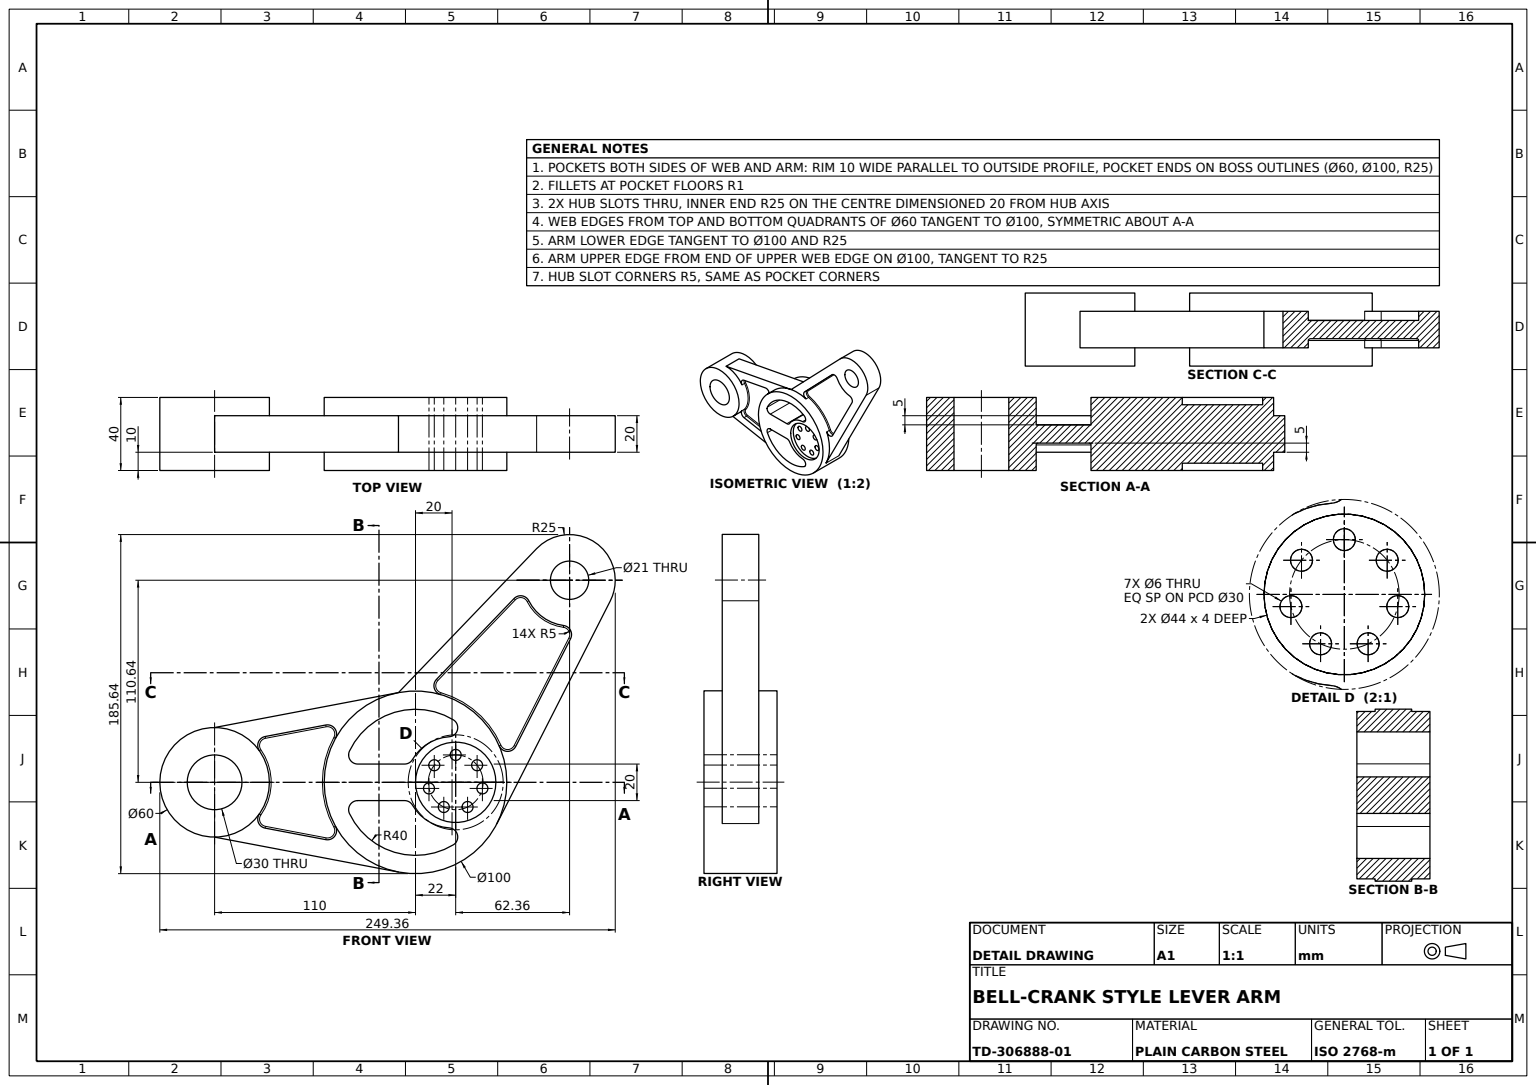
SolidWorks part; units mm, degrees
material "Plain Carbon Steel"
ref_plane "Front Plane" through (0, 0, 0) normal (0, 0, 1) x (1, 0, 0)
ref_plane "Top Plane" through (0, 0, 0) normal (0, 1, 0) x (1, 0, 0)
ref_plane "Right Plane" through (0, 0, 0) normal (1, 0, 0) x (0, 0, -1)
sketch "Lever Body Profile" plane through (0, 0, 0) normal (0, 0, 1) x (1, 0, 0)
  line L0 (0, 0) -> (-50, 0)
  line L1 (-5.9808, 10) -> (-31.6228, 10)
  line L2 (-5.9808, -10) -> (-31.6228, -10)
  line L4 (0, 10) -> (-50, 10) construction
  circle A0 centre (0, 0) radius 50
  arc A1 (20.7143, 34.2187) -> (-36.1403, 17.1429) centre (0, 0) ccw
  arc A4 (18.4375, 24.9511) -> (-1.6506, 12.5) centre (20, 0) ccw
  arc A5 (18.4375, 24.9511) -> (20.7143, 34.2187) centre (18.125, 29.9413) ccw
  arc A6 (18.4375, -24.9511) -> (20.7143, -34.2187) centre (18.125, -29.9413) cw
  arc A7 (-5.9808, -10) -> (-1.6506, -12.5) centre (-5.9808, -15) cw
  arc A8 (-5.9808, 10) -> (-1.6506, 12.5) centre (-5.9808, 15) ccw
  arc A9 (-31.6228, 10) -> (-36.1403, 17.1429) centre (-31.6228, 15) cw
  arc A10 (18.4375, -24.9511) -> (-1.6506, -12.5) centre (20, 0) cw
  arc A11 (-31.6228, -10) -> (-36.1403, -17.1429) centre (-31.6228, -15) ccw
  arc A12 (20.7143, -34.2187) -> (-36.1403, -17.1429) centre (0, 0) cw
  point P12 (0, -10)
  point P13 (-50, -10)
  dimension "D1" = 100
  dimension "D2" = 80
  dimension "D3" = 20
  dimension "D5" = 50
  dimension "D6" = 10
  dimension "D7" = 5
  dimension "D8" = 5
extrude "Lever Body" add sketch "Lever Body Profile" along normal blind 40
sketch "Front Pocket Profile" plane through (0, 0, 40) normal (0, 0, 1) x (1, 0, 0)
  line L0 (-5.9808, 10) -> (-31.6228, 10) construction
  circle A0 centre (22, 0) radius 22
  circle A2 centre (22, 15) radius 3
  circle A3 centre (33.7275, 9.3523) radius 3
  circle A4 centre (36.6239, -3.3378) radius 3
  circle A5 centre (28.5083, -13.5145) radius 3
  circle A6 centre (15.4917, -13.5145) radius 3
  circle A7 centre (7.3761, -3.3378) radius 3
  circle A8 centre (10.2725, 9.3523) radius 3
  dimension "D1" = 22
  dimension "D2" = 44
  dimension "D3" = 43.5164
  dimension "D4" = 6
  dimension "D5" = 7
  dimension "D6" = 46.4128
  dimension "D7" = 5
extrude "Front Pocket 4mm" cut sketch "Front Pocket Profile" against normal blind 4
sketch "Hub Through Cut Profile" plane through (0, 0, 40) normal (0, 0, 1) x (1, 0, 0)
  circle A0 centre (22, 15) radius 3
  circle A1 centre (33.7275, 9.3523) radius 3
  circle A2 centre (36.6239, -3.3378) radius 3
  circle A3 centre (28.5083, -13.5145) radius 3
  circle A4 centre (15.4917, -13.5145) radius 3
  circle A5 centre (7.3761, -3.3378) radius 3
  circle A6 centre (10.2725, 9.3523) radius 3
  circle A7 centre (22, 15) radius 3 construction
  dimension "D1" = 7
  dimension "D2" = 6
  dimension "D3" = 6.5083
extrude "Hub Through Cut" cut sketch "Hub Through Cut Profile" against normal blind 44
sketch "Rear Pocket Profile" plane through (0, 0, 0) normal (0, 0, -1) x (-1, 0, 0)
  line L0 (5.9808, 10) -> (31.6228, 10) construction
  circle A7 centre (-22, 0) radius 22
  circle A8 centre (-22, 15) radius 3
  circle A9 centre (-10.2725, 9.3523) radius 3
  circle A10 centre (-7.3761, -3.3378) radius 3
  circle A11 centre (-15.4917, -13.5145) radius 3
  circle A12 centre (-28.5083, -13.5145) radius 3
  circle A13 centre (-36.6239, -3.3378) radius 3
  circle A14 centre (-33.7275, 9.3523) radius 3
  dimension "D1" = 44
  dimension "D2" = 6
  dimension "D3" = 7
  dimension "D4" = 9.0267
  dimension "D5" = 11.9232
  dimension "D6" = 5
  dimension "D8" = 10
extrude "Rear Pocket 4mm" cut sketch "Rear Pocket Profile" against normal blind 4
sketch "Arm Boss Profile" plane through (0, 0, 40) normal (0, 0, 1) x (1, 0, 0)
  circle A0 centre (-110, 0) radius 15
  circle A1 centre (-110, 0) radius 30
  dimension "D1" = 60
  dimension "D2" = 30
  dimension "D3" = 110
  dimension "D4" = 73.8597
extrude "Arm Boss" add sketch "Arm Boss Profile" against normal blind 40 separate body
sketch "Web Arm Profile" plane through (0, 0, 40) normal (0, 0, 1) x (1, 0, 0)
  line L0 (22, 15) -> (22, 0)
  line L1 (-5.9808, 10) -> (-31.6228, 10) construction
  circle A0 centre (84.359, 110.6361) radius 10.5
  circle A1 centre (84.359, 110.6361) radius 25
  dimension "D1" = 21
  dimension "D2" = 50
  dimension "D3" = 127
  dimension "D4" = 62.359
  dimension "D5" = 100.6361
extrude "Triangular Web Arm" add sketch "Web Arm Profile" against normal blind 40 separate body contours A1 A0
ref_plane "Plane1" through (0, 0, 20) normal (0, 0, 1) x (1, 0, 0)
sketch "Front Hub Boss Profile" plane through (0, 0, 20) normal (0, 0, 1) x (1, 0, 0)
  line L0 (-110, 30) -> (-9.3304, 49.1217)
  line L1 (-110, -30) -> (-9.3304, -49.1217)
  line L2 (-9.3304, 49.1217) -> (66.3221, 127.9471)
  line L3 (106.6394, 99.2967) -> (44.5608, -22.6789)
  line L4 (11.4718, 56.3547) -> (53.9518, 100.6162)
  line L5 (84.8981, 78.625) -> (54.8924, 19.668)
  line L6 (-110, 0) -> (0, 0)
  line L7 (-2.1157, 42.1973) -> (73.5368, 121.0227) construction
  line L8 (97.7273, 103.8325) -> (35.6487, -18.1431) construction
  line L9 (-82.3262, 25.0777) -> (-49.1455, 31.3802)
  line L10 (-82.3262, -25.0777) -> (-49.1455, -31.3802)
  line L11 (-108.1339, 20.1757) -> (-7.4644, 39.2974) construction
  arc A0 (-110, 30) -> (-110, -30) centre (-110, 0) cw
  circle A1 centre (-110, 0) radius 30 construction
  circle A2 centre (0, 0) radius 50 construction
  circle A3 centre (0, 0) radius 50
  circle A4 centre (84.359, 110.6361) radius 25 construction
  arc A5 (66.3221, 127.9471) -> (106.6394, 99.2967) centre (84.359, 110.6361) ccw
  arc A6 (11.4718, 56.3547) -> (13.7084, 48.0841) centre (15.0792, 52.8925) ccw
  arc A7 (45.8512, 19.9417) -> (54.8924, 19.668) centre (50.4363, 21.9359) ccw
  arc A8 (53.9518, 100.6162) -> (62.0258, 99.401) centre (57.5591, 97.154) cw
  arc A9 (81.0949, 85.8501) -> (84.8981, 78.625) centre (80.442, 80.8929) cw
  arc A10 (-82.3262, 25.0777) -> (-85.4799, 17.2847) centre (-81.3932, 20.1655) ccw
  arc A11 (-49.1455, 31.3802) -> (-43.8295, 24.0619) centre (-48.2125, 26.4681) cw
  arc A12 (-49.1455, -31.3802) -> (-43.8295, -24.0619) centre (-48.2125, -26.4681) ccw
  arc A13 (-82.3262, -25.0777) -> (-85.4799, -17.2847) centre (-81.3932, -20.1655) cw
  dimension "D1" = 30
  dimension "D2" = 100
  dimension "D6" = 5
  dimension "D7" = 5
  dimension "D8" = 5
  dimension "D9" = 5
  dimension "D11" = 5
  dimension "D12" = 5
  dimension "D10" = 10
  dimension "D4" = 10
  dimension "D5" = 10
extrude "Front Hub Boss" add sketch "Front Hub Boss Profile" along normal mid plane 20 contours L9 A11 A3 L0 A0 A10 | L10 A13 A0 L1 A3 A12 | L4 A8 A5 L2 A3 A6 | A5 A9 L5 A7 A3 L3
ref_plane "Plane2" through (0, 0, 20) normal (0, 0, 1) x (1, 0, 0)
sketch "Rear Hub Flange Profile" plane through (0, 0, 20) normal (0, 0, 1) x (1, 0, 0)
  line L0 (-82.3262, 25.0777) -> (-49.1455, 31.3802)
  line L1 (-82.3262, -25.0777) -> (-49.1455, -31.3802)
  line L2 (11.4718, 56.3547) -> (53.9518, 100.6162)
  line L3 (84.8981, 78.625) -> (54.8924, 19.668)
  arc A0 (-85.4799, 17.2847) -> (-82.3262, 25.0777) centre (-81.3932, 20.1655) cw
  arc A1 (-49.1455, 31.3802) -> (-43.8295, 24.0619) centre (-48.2125, 26.4681) cw
  arc A2 (-85.4799, -17.2847) -> (-82.3262, -25.0777) centre (-81.3932, -20.1655) ccw
  arc A3 (-49.1455, -31.3802) -> (-43.8295, -24.0619) centre (-48.2125, -26.4681) ccw
  arc A4 (11.4718, 56.3547) -> (13.7084, 48.0841) centre (15.0792, 52.8925) ccw
  arc A5 (53.9518, 100.6162) -> (62.0258, 99.401) centre (57.5591, 97.154) cw
  circle A6 centre (84.359, 110.6361) radius 25 construction
  arc A7 (66.3221, 127.9471) -> (62.0258, 99.401) centre (84.359, 110.6361) ccw construction
  arc A8 (81.0949, 85.8501) -> (84.8981, 78.625) centre (80.442, 80.8929) cw
  arc A9 (45.8512, 19.9417) -> (54.8924, 19.668) centre (50.4363, 21.9359) ccw
  arc A10 (-43.8295, 24.0619) -> (-43.8295, -24.0619) centre (0, 0) ccw
  arc A11 (13.7084, 48.0841) -> (45.8512, 19.9417) centre (0, 0) cw
  arc A12 (-85.4799, 17.2847) -> (-85.4799, -17.2847) centre (-110, 0) cw
  arc A13 (62.0258, 99.401) -> (81.0949, 85.8501) centre (84.359, 110.6361) ccw
extrude "Rear Hub Flange" add sketch "Rear Hub Flange Profile" along normal mid plane 10
fillet "Hub Edge Fillet R1 A" radius 1 8 edges at (-44.1671, 29.4066, 25) (-50, 0, 25) (-44.1671, -29.4066, 25) (-65.7359, -28.229, 25) (-86.028, -22.0412, 25) (-80, 0, 25) (-86.028, 22.0412, 25) (-65.7359, 28.229, 25)
fillet "Hub Edge Fillet R1 B" radius 1 8 edges at (58.3033, 102.0983, 25) (69.8775, 90.2575, 25) (84.8665, 83.2219, 25) (69.8952, 49.1465, 25) (50.285, 16.9382, 25) (32.9368, 37.6187, 25) (10.2526, 51.5873, 25) (32.7118, 78.4855, 25)
sketch "Web Arm Cut A Profile" plane through (0, 0, 40) normal (0, 0, 1) x (1, 0, 0)
  circle A0 centre (84.359, 110.6361) radius 10.5
  circle A1 centre (84.359, 110.6361) radius 25
  dimension "D1" = 21
  dimension "D2" = 50
extrude "Web Arm Cut A" cut sketch "Web Arm Cut A Profile" against normal blind 10
sketch "Web Arm Cut B Profile" plane through (0, 0, 0) normal (0, 0, -1) x (-1, 0, 0)
  circle A0 centre (-84.359, 110.6361) radius 10.5
  circle A1 centre (-84.359, 110.6361) radius 25
  dimension "D1" = 21
  dimension "D2" = 50
extrude "Web Arm Cut B" cut sketch "Web Arm Cut B Profile" against normal blind 10
